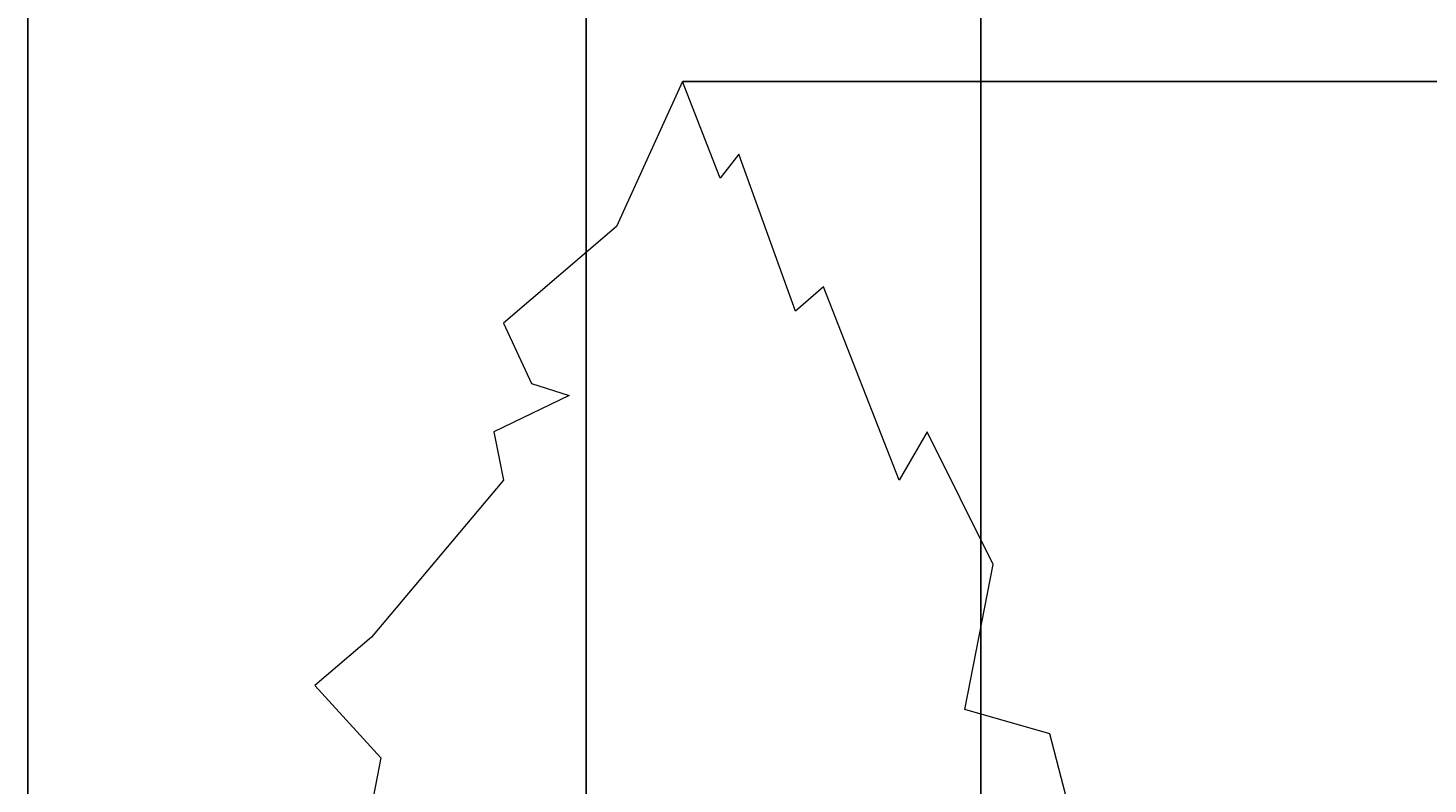
# Model space of a CAD drawing. Units: inches. Extents: x -26 to 776, y -22 to 650.
# Tile 58 of 62: x 426 to 601, y 321 to 415. Entities that reach past the tile are written whole.
import ezdxf

# ---------------------------------------------------------------- set-up
doc = ezdxf.new("R2010")
doc.units = ezdxf.units.IN
doc.header["$MEASUREMENT"] = 0
doc.layers.add('A-ANNO-DIMS', color=2, linetype='Continuous', lineweight=18)
doc.layers.add('L-PLNT-TREE', color=94, linetype='Continuous', lineweight=18)
doc.styles.get("Standard").update_dxf_attribs({"font": 'arial.ttf'})
doc.dimstyles.get("Standard").update_dxf_attribs({"dimtxt": 0.5625, "dimasz": 0.18, "dimexe": 0.18, "dimexo": 0.0625, "dimgap": 0.09, "dimtad": 0, "dimtih": 1, "dimtoh": 1, "dimdec": 4, "dimzin": 0, "dimdsep": 46, "dimlunit": 4, "dimtxsty": 'Standard', "dimcen": 0.09, "dimadec": 0, "dimazin": 0, "dimtfac": 1, "dimtdec": 4, "dimtofl": 0, "dimtmove": 0, "dimatfit": 3, "dimfxl": 1, "dimtolj": 1, "dimtzin": 0, "dimarcsym": 0})

# ---------------------------------------------------------------- blocks, each defined once
blk = doc.blocks.new('Tree - type 2 deciduous elevation')
blk.add_lwpolyline([(22.551, 140.825), (19.675, 151.884), (14.499, 153.359), (16.224, 162.207), (12.199, 170.317), (10.473, 167.368), (5.872, 179.165), (4.147, 177.69), (0.696, 187.275), (-0.454, 185.8), (-2.754, 191.699), (-6.78, 182.851), (-13.682, 176.953), (-11.956, 173.266), (-9.656, 172.529), (-14.257, 170.317), (-13.682, 167.368), (-21.733, 157.783), (-25.184, 154.834), (-21.158, 150.41), (-21.733, 147.461)])
blk = doc.blocks.new('*D20')
at = {"layer": 'A-ANNO-DIMS', "color": 0, "lineweight": -2, "transparency": 16777216}
for p, q in [((425.81, 455.47), (775.34, 455.47)), ((775.16, 455.29), (775.16, 235.85)), ((775.16, 15.66), (775.16, 235.1)), ((425.81, 15.48), (775.34, 15.48))]:
    blk.add_line(p, q, dxfattribs=at)
at = {"layer": 'A-ANNO-DIMS', "color": 0, "transparency": 16777216}
for points in [[(775.13, 455.29), (775.19, 455.29), (775.16, 455.47)], [(775.13, 15.66), (775.19, 15.66), (775.16, 15.48)]]:
    blk.add_solid(points, dxfattribs=at)
at = {"layer": 'Defpoints', "color": 0, "transparency": 16777216}
for p in [(425.74, 455.47), (775.16, 455.47), (425.74, 15.48)]:
    blk.add_point(p, dxfattribs=at)
at = {"layer": 'A-ANNO-DIMS', "color": 0, "transparency": 16777216, "insert": (775.16, 235.48), "char_height": 0.562, "attachment_point": 5}
blk.add_mtext('\\A1;440', dxfattribs=at)
blk = doc.blocks.new('*D39')
at = {"layer": 'A-ANNO-DIMS', "color": 0, "lineweight": -2, "transparency": 16777216}
for p, q in [((289.24, 15.54), (289.24, 649.86)), ((289.42, 649.68), (356.48, 649.68)), ((425.56, 649.68), (358.51, 649.68)), ((425.74, 15.54), (425.74, 649.86))]:
    blk.add_line(p, q, dxfattribs=at)
at = {"layer": 'A-ANNO-DIMS', "color": 0, "transparency": 16777216}
for points in [[(289.42, 649.71), (289.42, 649.65), (289.24, 649.68)], [(425.56, 649.71), (425.56, 649.65), (425.74, 649.68)]]:
    blk.add_solid(points, dxfattribs=at)
at = {"layer": 'Defpoints', "color": 0, "transparency": 16777216}
for p in [(425.74, 649.68), (289.24, 15.48), (425.74, 15.48)]:
    blk.add_point(p, dxfattribs=at)
at = {"layer": 'A-ANNO-DIMS', "color": 0, "transparency": 16777216, "insert": (357.49, 649.68), "char_height": 0.562, "attachment_point": 5}
blk.add_mtext('\\A1;136.5', dxfattribs=at)
blk = doc.blocks.new('*D40')
at = {"layer": 'A-ANNO-DIMS', "color": 0, "lineweight": -2, "transparency": 16777216}
for p, q in [((425.74, 15.54), (425.74, 649.86)), ((425.92, 649.68), (459.65, 649.68)), ((495.45, 649.68), (461.73, 649.68)), ((495.63, 15.54), (495.63, 649.86))]:
    blk.add_line(p, q, dxfattribs=at)
at = {"layer": 'A-ANNO-DIMS', "color": 0, "transparency": 16777216}
for points in [[(425.92, 649.71), (425.92, 649.65), (425.74, 649.68)], [(495.45, 649.71), (495.45, 649.65), (495.63, 649.68)]]:
    blk.add_solid(points, dxfattribs=at)
at = {"layer": 'Defpoints', "color": 0, "transparency": 16777216}
for p in [(495.63, 649.68), (425.74, 15.48), (495.63, 15.48)]:
    blk.add_point(p, dxfattribs=at)
at = {"layer": 'A-ANNO-DIMS', "color": 0, "transparency": 16777216, "insert": (460.69, 649.68), "char_height": 0.562, "attachment_point": 5}
blk.add_mtext('\\A1;69.89', dxfattribs=at)
blk = doc.blocks.new('*D45')
at = {"layer": 'A-ANNO-DIMS', "color": 0, "lineweight": -2, "transparency": 16777216}
for p, q in [((507.74, 408.64), (775.34, 408.64)), ((775.16, 408.46), (775.16, 212.44)), ((775.16, 15.66), (775.16, 211.68)), ((586, 15.48), (775.34, 15.48))]:
    blk.add_line(p, q, dxfattribs=at)
at = {"layer": 'A-ANNO-DIMS', "color": 0, "transparency": 16777216}
for points in [[(775.13, 408.46), (775.19, 408.46), (775.16, 408.64)], [(775.13, 15.66), (775.19, 15.66), (775.16, 15.48)]]:
    blk.add_solid(points, dxfattribs=at)
at = {"layer": 'Defpoints', "color": 0, "transparency": 16777216}
for p in [(507.68, 408.64), (775.16, 408.64), (585.94, 15.48)]:
    blk.add_point(p, dxfattribs=at)
at = {"layer": 'A-ANNO-DIMS', "color": 0, "transparency": 16777216, "insert": (775.16, 212.06), "char_height": 0.562, "attachment_point": 5}
blk.add_mtext('\\A1;393.16', dxfattribs=at)
blk = doc.blocks.new('*D48')
at = {"layer": 'A-ANNO-DIMS', "color": 0, "lineweight": -2, "transparency": 16777216}
for p, q in [((545.03, 67.41), (545.03, 649.86)), ((545.21, 649.68), (640.88, 649.68)), ((738.57, 649.68), (642.9, 649.68)), ((738.75, 50.91), (738.75, 649.86))]:
    blk.add_line(p, q, dxfattribs=at)
at = {"layer": 'A-ANNO-DIMS', "color": 0, "transparency": 16777216}
for points in [[(545.21, 649.71), (545.21, 649.65), (545.03, 649.68)], [(738.57, 649.71), (738.57, 649.65), (738.75, 649.68)]]:
    blk.add_solid(points, dxfattribs=at)
at = {"layer": 'Defpoints', "color": 0, "transparency": 16777216}
for p in [(738.75, 649.68), (545.03, 67.35), (738.75, 50.85)]:
    blk.add_point(p, dxfattribs=at)
at = {"layer": 'A-ANNO-DIMS', "color": 0, "transparency": 16777216, "insert": (641.89, 649.68), "char_height": 0.562, "attachment_point": 5}
blk.add_mtext('\\A1;193.7', dxfattribs=at)

msp = doc.modelspace()

# ---------------------------------------------------------------- block references
at = {"layer": 'L-PLNT-TREE', "xscale": 2.050905272406618, "yscale": 2.050905272406618, "zscale": 2.050905272406618}
msp.add_blockref('Tree - type 2 deciduous elevation', (513.3241, 15.4824), dxfattribs=at)

# ---------------------------------------------------------------- dimensions: what is measured, and where the dimension line sits
at = {"layer": 'A-ANNO-DIMS'}
for base, p1, p2, override, picture, middle in [((425.7434, 649.6763), (289.2424, 15.4824), (425.7434, 15.4824), {"dimdec": 1, "dimlfac": 1, "dimrnd": 0, "dimzin": 0, "dimdsep": 46, "dimlunit": 2}, '*D39', (357.4929, 649.6763)), ((495.6309, 649.6763), (425.7434, 15.4824), (495.6309, 15.4824), {"dimdec": 2, "dimlfac": 1, "dimrnd": 0, "dimzin": 0, "dimdsep": 46, "dimlunit": 2}, '*D40', (460.6872, 649.6763)), ((738.7503, 649.6763), (545.0331, 67.3523), (738.7503, 50.8482), {"dimdec": 1, "dimlfac": 1, "dimrnd": 0, "dimzin": 0, "dimdsep": 46, "dimlunit": 2}, '*D48', (641.8917, 649.6763))]:
    dim = msp.add_linear_dim(base=base, p1=p1, p2=p2, dimstyle='Standard', override=override, dxfattribs=at)
    dim.commit()
    dim.dimension.update_dxf_attribs({"geometry": picture, "text_midpoint": middle})
for base, p1, p2, override, picture, middle in [((775.1553, 455.4717), (425.7434, 15.4824), (425.7434, 455.4717), {"dimdec": 0, "dimlfac": 1, "dimrnd": 0, "dimzin": 0, "dimdsep": 46, "dimlunit": 2}, '*D20', (775.1553, 235.477)), ((775.1553, 408.6389), (585.9354, 15.4824), (507.6759, 408.6389), {"dimdec": 2, "dimlfac": 1, "dimrnd": 0, "dimzin": 0, "dimdsep": 46, "dimlunit": 2}, '*D45', (775.1553, 212.0606))]:
    dim = msp.add_linear_dim(base=base, p1=p1, p2=p2, angle=90, dimstyle='Standard', override=override, dxfattribs=at)
    dim.commit()
    dim.dimension.update_dxf_attribs({"geometry": picture, "text_midpoint": middle})

doc.saveas('drawing.dxf')
